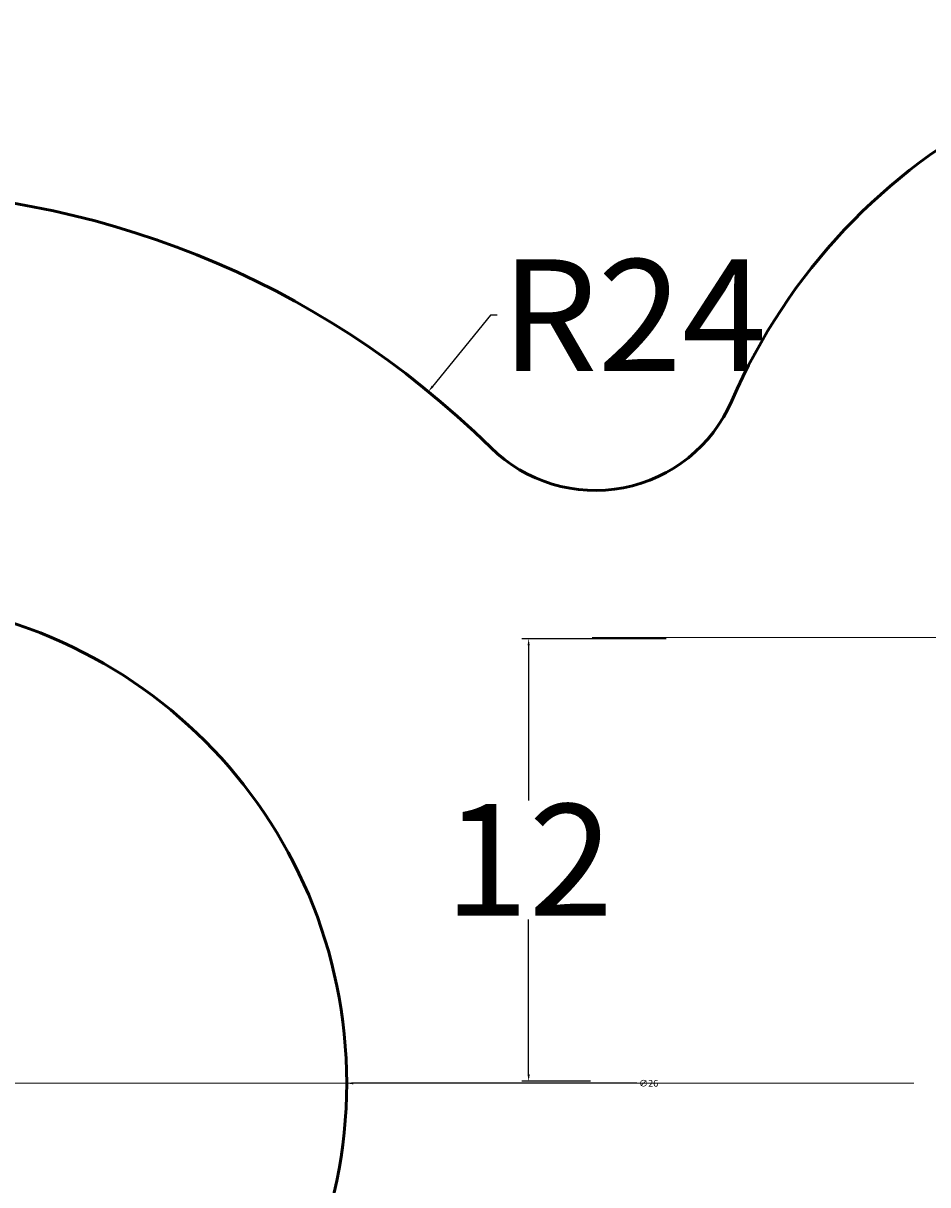
# Model space of a CAD drawing. Units: millimetres. Extents: x -50 to 109, y -46 to 152.
# Tile 16 of 18: x 37 to 62, y 100 to 131. Entities that reach past the tile are written whole.
import ezdxf

# ---------------------------------------------------------------- set-up
doc = ezdxf.new("R2010")
doc.units = ezdxf.units.MM
doc.header["$MEASUREMENT"] = 0
doc.linetypes.add('CENTER', pattern=[50.8, 31.75, -6.35, 6.35, -6.35])
for name, color, linetype, lineweight in [('M-CNTR', 1, 'CENTER', 18), ('M-DIMS', 2, 'Continuous', 25), ('M-OUTL', 7, 'Continuous', 50)]:
    doc.layers.add(name, color=color, linetype=linetype, lineweight=lineweight)
doc.styles.get("Standard").update_dxf_attribs({"font": 'arial.ttf'})
doc.dimstyles.get("Standard").update_dxf_attribs({"dimtxt": 0.18, "dimasz": 0.18, "dimexe": 0.18, "dimexo": 0.0625, "dimgap": 0.09, "dimtad": 0, "dimtih": 1, "dimtoh": 1, "dimdec": 4, "dimzin": 0, "dimdsep": 46, "dimtxsty": 'Standard', "dimcen": 0.09, "dimadec": 0, "dimazin": 0, "dimtfac": 1, "dimtdec": 4, "dimtofl": 0, "dimtmove": 0, "dimatfit": 3, "dimfxl": 1, "dimtolj": 1, "dimtzin": 0, "dimarcsym": 0})

# ---------------------------------------------------------------- blocks, each defined once
blk = doc.blocks.new('*U3')
at = {"layer": 'M-CNTR', "color": 0, "transparency": 16777216}
blk.add_line((2.6, 0), (28.243, 0), dxfattribs=at)
blk = doc.blocks.new('*U4')
at = {"layer": 'M-CNTR', "color": 0, "transparency": 16777216}
for p, q in [((0, 1.8), (0, 9.12)), ((-18.399, 0), (-1.8, 0)), ((1.8, 0), (9.12, 0)), ((0, -9.12), (0, -1.8))]:
    blk.add_line(p, q, dxfattribs=at)
at = {"layer": 'M-CNTR', "color": 0, "linetype": 'Continuous', "transparency": 16777216}
for p, q in [((0, -0.9), (0, 0.9)), ((-0.9, 0), (0.9, 0))]:
    blk.add_line(p, q, dxfattribs=at)
blk = doc.blocks.new('*D7')
at = {"layer": 'Defpoints', "color": 0, "transparency": 16777216}
for p in [(70.892, 150.415), (-5.074, 114.299), (70.892, 114.299)]:
    blk.add_point(p, dxfattribs=at)
at = {"layer": 'M-DIMS', "color": 0, "lineweight": -2, "transparency": 16777216}
for p, q in [((-5.074, 114.361), (-5.074, 150.595)), ((-4.894, 150.415), (30.684, 150.415)), ((70.712, 150.415), (35.134, 150.415)), ((70.892, 114.361), (70.892, 150.595))]:
    blk.add_line(p, q, dxfattribs=at)
at = {"layer": 'M-DIMS', "color": 0, "transparency": 16777216}
for points in [[(-4.894, 150.445), (-4.894, 150.385), (-5.074, 150.415)], [(70.712, 150.445), (70.712, 150.385), (70.892, 150.415)]]:
    blk.add_solid(points, dxfattribs=at)
at = {"layer": 'M-DIMS', "color": 0, "transparency": 16777216, "insert": (32.909, 150.415), "char_height": 0.18, "attachment_point": 5}
blk.add_mtext('\\A1;{\\H16.66667x;76}', dxfattribs=at)
blk = doc.blocks.new('*D9')
at = {"layer": 'Defpoints', "color": 0, "transparency": 16777216}
for p in [(48.315, 120.834), (33.155, 102.229)]:
    blk.add_point(p, dxfattribs=at)
at = {"layer": 'M-DIMS', "color": 0, "lineweight": -2, "transparency": 16777216}
for p, q in [((49.988, 122.887), (48.429, 120.974)), ((50.168, 122.887), (49.988, 122.887)), ((33.065, 102.229), (33.245, 102.229)), ((33.155, 102.139), (33.155, 102.319))]:
    blk.add_line(p, q, dxfattribs=at)
at = {"layer": 'M-DIMS', "color": 0, "transparency": 16777216}
blk.add_solid([(48.406, 120.993), (48.452, 120.955), (48.315, 120.834)], dxfattribs=at)
at = {"layer": 'M-DIMS', "color": 0, "transparency": 16777216, "insert": (53.836, 122.887), "char_height": 0.18, "attachment_point": 5}
blk.add_mtext('\\A1;{\\H16.66667x;R24}', dxfattribs=at)
blk = doc.blocks.new('*D12')
at = {"layer": 'Defpoints', "color": 0, "transparency": 16777216}
for p in [(51.01, 114.194), (54.766, 114.194), (52.732, 102.31)]:
    blk.add_point(p, dxfattribs=at)
at = {"layer": 'M-DIMS', "color": 0, "lineweight": -2, "transparency": 16777216}
for p, q in [((54.704, 114.194), (50.83, 114.194)), ((51.01, 114.014), (51.01, 109.848)), ((51.01, 102.49), (51.01, 106.656)), ((52.669, 102.31), (50.83, 102.31))]:
    blk.add_line(p, q, dxfattribs=at)
at = {"layer": 'M-DIMS', "color": 0, "transparency": 16777216}
for points in [[(50.98, 114.014), (51.04, 114.014), (51.01, 114.194)], [(50.98, 102.49), (51.04, 102.49), (51.01, 102.31)]]:
    blk.add_solid(points, dxfattribs=at)
at = {"layer": 'M-DIMS', "color": 0, "transparency": 16777216, "insert": (51.01, 108.252), "char_height": 0.18, "attachment_point": 5}
blk.add_mtext('\\A1;{\\H16.66667x;12}', dxfattribs=at)
blk = doc.blocks.new('*D30')
at = {"layer": 'Defpoints', "color": 0, "transparency": 16777216}
for p in [(20.119, 102.25), (46.119, 102.251)]:
    blk.add_point(p, dxfattribs=at)
at = {"layer": 'M-DIMS', "color": 0, "lineweight": -2, "transparency": 16777216}
for p, q in [((33.029, 102.251), (33.209, 102.251)), ((33.119, 102.161), (33.119, 102.341)), ((53.919, 102.251), (46.299, 102.251))]:
    blk.add_line(p, q, dxfattribs=at)
at = {"layer": 'M-DIMS', "color": 0, "transparency": 16777216}
blk.add_solid([(46.299, 102.281), (46.299, 102.221), (46.119, 102.251)], dxfattribs=at)
at = {"layer": 'M-DIMS', "color": 0, "transparency": 16777216, "insert": (54.236, 102.251), "char_height": 0.18, "attachment_point": 5}
blk.add_mtext('\\A1;∅26', dxfattribs=at)

msp = doc.modelspace()

# ---------------------------------------------------------------- linework, layer by layer
at = {"layer": 'M-OUTL'}
msp.add_circle((33.11888, 102.25066), 13, dxfattribs=at)
for centre, radius, start, end in [((71.1447, 114.20575), 16, 359.978447, 156.508505), ((33.15497, 102.22852), 24, 45.437177, 134.672076), ((52.80232, 122.17801), 4, 225.437177, 336.508505)]:
    msp.add_arc(centre, radius, start, end, dxfattribs=at)

# ---------------------------------------------------------------- block references
at = {"layer": 'M-CNTR'}
for name, p in [('*U3', (33.11888, 102.25066)), ('*U4', (71.11949, 114.23094))]:
    msp.add_blockref(name, p, dxfattribs=at)

# ---------------------------------------------------------------- dimensions: what is measured, and where the dimension line sits
at = {"layer": 'M-DIMS'}
dim = msp.add_linear_dim(base=(70.89158, 150.41471), p1=(-5.07376, 114.29893), p2=(70.89158, 114.29893), text='{\\H16.66667x;76}', dimstyle='Standard', override={"dimclrd": 0, "dimclre": 0, "dimclrt": 0}, dxfattribs=at)
dim.commit()
dim.dimension.update_dxf_attribs({"geometry": '*D7', "text_midpoint": (32.90891, 150.41471)})
dim = msp.add_radius_dim(center=(33.15497, 102.22852), mpoint=(48.3151, 120.83418), text='{\\H16.66667x;R24}', dimstyle='Standard', override={"dimclrd": 0, "dimclre": 0, "dimclrt": 0}, dxfattribs=at)
dim.commit()
dim.dimension.update_dxf_attribs({"geometry": '*D9', "text_midpoint": (53.83605, 122.88721), "dimtype": 164})
dim = msp.add_linear_dim(base=(51.01033, 114.19428), p1=(52.73186, 102.30971), p2=(54.76639, 114.19428), angle=90, text='{\\H16.66667x;12}', dimstyle='Standard', override={"dimclrd": 0, "dimclre": 0, "dimclrt": 0}, dxfattribs=at)
dim.commit()
dim.dimension.update_dxf_attribs({"geometry": '*D12', "text_midpoint": (51.01033, 108.252)})
dim = msp.add_diameter_dim_2p(p1=(20.11888, 102.25033), p2=(46.11888, 102.251), dimstyle='Standard', override={"dimdec": 0, "dimlfac": 1, "dimrnd": 0, "dimzin": 0, "dimdsep": 46, "dimlunit": 2}, dxfattribs=at)
dim.commit()
dim.dimension.update_dxf_attribs({"geometry": '*D30', "text_midpoint": (53.91888, 102.2512), "dimtype": 163})

doc.saveas('drawing.dxf')
